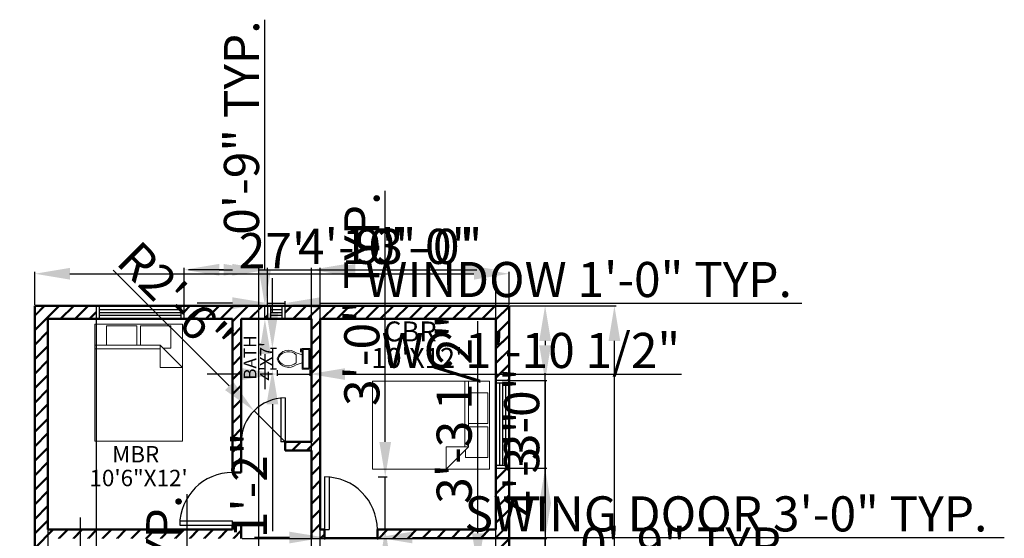
# Model space of a CAD drawing. Units: inches. Extents: x -584 to 444, y 228 to 1001.
# Tile 5 of 5: x -228 to 444, y 647 to 1001. Entities that reach past the tile are written whole.
import ezdxf

# ---------------------------------------------------------------- set-up
doc = ezdxf.new("R2010")
doc.units = ezdxf.units.IN
for name, color, linetype, lineweight in [('A-ANNO-DIMS', 2, 'Continuous', 18), ('A-AREA-IDEN', 7, 'Continuous', 25), ('A-DOOR', 3, 'Continuous', 25), ('A-FLOR-FIXT', 9, 'Continuous', 18), ('A-FURN', 8, 'Continuous', 18), ('A-GLAZ', 4, 'Continuous', 25), ('A-WALL', 7, 'Continuous', 50), ('A-WALL-PATT', 3, 'Continuous', 13)]:
    doc.layers.add(name, color=color, linetype=linetype, lineweight=lineweight)
doc.styles.get("Standard").update_dxf_attribs({"font": 'arial.ttf'})
doc.dimstyles.new('ISO-25', dxfattribs={"dimtxt": 24, "dimasz": 24, "dimexe": 1.25, "dimexo": 0.625, "dimtad": 1, "dimdec": 1, "dimlunit": 3, "dimtxsty": 'Standard', "dimcen": 2.5, "dimadec": 0, "dimazin": 0, "dimtfac": 1, "dimtdec": 1, "dimtmove": 0, "dimatfit": 3, "dimfxl": 1, "dimarcsym": 0})

# ---------------------------------------------------------------- blocks, each defined once
blk = doc.blocks.new('Bed - Queen')
for p, q in [((0, -80.00003), (0, 0)), ((0, 0), (59.99999, 0)), ((59.99999, 0), (59.99999, -80.00003)), ((7.99999, -1.2), (28.79998, -1.2)), ((7.99999, -14.4), (7.99999, -1.2)), ((28.79998, -1.2), (28.79998, -14.4)), ((31.19999, -1.2), (51.99999, -1.2)), ((31.19999, -14.4), (31.19999, -1.2)), ((51.99999, -1.2), (51.99999, -16.4)), ((0, -14.4), (44.8, -14.4)), ((44.8, -16.8), (0, -16.8)), ((59.99999, -29.6), (44.8, -14.4)), ((44.8, -14.4), (44.8, -29.6)), ((51.99999, -16.4), (46.79936, -16.4)), ((44.8, -29.6), (59.99999, -29.6)), ((59.99999, -80.00003), (0, -80.00003))]:
    blk.add_line(p, q)
blk = doc.blocks.new('Toilet - top')
for p, q in [((-10, -8.5), (-8, -8.5)), ((-10, -9.5), (-10, -8.5)), ((-7, -9.5), (-10, -9.5)), ((-8, -8.5), (-8, -8)), ((-7, -8), (-7, -9.5)), ((-4, -8), (-6, -14)), ((4, -8), (6, -14)), ((9.5, -6), (9.5, -2)), ((4, -14), (-4, -14))]:
    blk.add_line(p, q)
blk.add_lwpolyline([(10.5, -8), (10.5, 0), (-10.5, 0), (-10.5, -8)], close=True)
for points in [[(-9.5, -2), (-9.5, -6)], [(8.5, -1), (-8.5, -1)], [(-8.5, -7), (8.5, -7)]]:
    blk.add_lwpolyline(points)
for centre, radius, start, end in [((-8.62, -1.88), 0.884, 81.8699, 188.1301), ((-8.62, -6.12), 0.884, 171.8699, 278.1301), ((8.62, -1.88), 0.884, 351.8699, 98.1301), ((8.62, -6.12), 0.884, 261.8699, 8.1301), ((3.52, -21.58), 12.17, 141.46911, 247.97143), ((4.2, -21.82), 11.33, 136.36773, 238.94682), ((-3.52, -21.58), 12.17, 292.02843, 38.53071), ((-4.2, -21.82), 11.33, 301.05301, 43.63209), ((0, -27.88), 4, 245.73182, 294.26817), ((0, -29), 4, 254.86053, 285.13947)]:
    blk.add_arc(centre, radius, start, end)
blk = doc.blocks.new('*D6')
at = {"layer": 'A-ANNO-DIMS', "color": 0, "lineweight": -2, "transparency": 16777216}
for p, q in [((-218.14, 806.16), (-218.14, 828.68)), ((-194.14, 827.43), (81.86, 827.43)), ((105.86, 806.16), (105.86, 828.68))]:
    blk.add_line(p, q, dxfattribs=at)
at = {"layer": 'A-ANNO-DIMS', "color": 0, "transparency": 16777216}
for points in [[(-194.14, 831.43), (-194.14, 823.43), (-218.14, 827.43)], [(81.86, 831.43), (81.86, 823.43), (105.86, 827.43)]]:
    blk.add_solid(points, dxfattribs=at)
at = {"layer": 'Defpoints', "color": 0, "transparency": 16777216}
for p in [(105.86, 827.43), (-218.14, 805.54), (105.86, 805.54)]:
    blk.add_point(p, dxfattribs=at)
at = {"layer": 'A-ANNO-DIMS', "color": 0, "transparency": 16777216, "insert": (-56.14, 840.11), "char_height": 24, "attachment_point": 5}
blk.add_mtext("27'", dxfattribs=at)
blk = doc.blocks.new('*D7')
at = {"layer": 'A-ANNO-DIMS', "color": 0, "lineweight": -2, "transparency": 16777216}
for p, q in [((106.48, 805.54), (179.05, 805.54)), ((177.8, 409.54), (177.8, 781.54)), ((106.48, 385.54), (179.05, 385.54))]:
    blk.add_line(p, q, dxfattribs=at)
at = {"layer": 'A-ANNO-DIMS', "color": 0, "transparency": 16777216}
for points in [[(173.8, 781.54), (181.8, 781.54), (177.8, 805.54)], [(173.8, 409.54), (181.8, 409.54), (177.8, 385.54)]]:
    blk.add_solid(points, dxfattribs=at)
at = {"layer": 'Defpoints', "color": 0, "transparency": 16777216}
for p in [(105.86, 805.54), (177.8, 805.54), (105.86, 385.54)]:
    blk.add_point(p, dxfattribs=at)
at = {"layer": 'A-ANNO-DIMS', "color": 0, "transparency": 16777216, "insert": (164.91, 595.54), "char_height": 24, "attachment_point": 5, "rotation": 90}
blk.add_mtext("35'", dxfattribs=at)
blk = doc.blocks.new('WIN-60IN')
for p, q in [((60, 9), (0, 9)), ((0, 9), (0, 0)), ((2, 9), (2, 0)), ((58, 0), (58, 9)), ((60, 0), (60, 9)), ((0, 0), (60, 0)), ((2, 6.5), (58, 6.5)), ((2, 4.5), (58, 4.5)), ((2, 2.5), (58, 2.5))]:
    blk.add_line(p, q)
blk = doc.blocks.new('WIN-12IN')
for p, q in [((12, 9), (0, 9)), ((0, 9), (0, 0)), ((2, 9), (2, 0)), ((10, 0), (10, 9)), ((12, 0), (12, 9)), ((0, 0), (12, 0)), ((2, 6.5), (10, 6.5)), ((2, 4.5), (10, 4.5)), ((2, 2.5), (10, 2.5))]:
    blk.add_line(p, q)
blk = doc.blocks.new('DOOR-SWING-36IN')
for p, q in [((0, 36), (0, 0)), ((3, 36), (3, 0)), ((0, 0), (3, 0))]:
    blk.add_line(p, q)
blk.add_arc((0, 0), 36, 0, 90)
blk = doc.blocks.new('*D12')
at = {"layer": 'A-ANNO-DIMS', "color": 0, "lineweight": -2, "transparency": 16777216}
for p, q in [((72.86, 626.04), (48.86, 626.04)), ((96.86, 617.66), (96.86, 627.29)), ((96.86, 626.04), (105.86, 626.04)), ((105.86, 617.66), (105.86, 627.29)), ((129.86, 626.04), (301.4, 626.04))]:
    blk.add_line(p, q, dxfattribs=at)
at = {"layer": 'A-ANNO-DIMS', "color": 0, "transparency": 16777216}
for points in [[(72.86, 630.04), (72.86, 622.04), (96.86, 626.04)], [(129.86, 630.04), (129.86, 622.04), (105.86, 626.04)]]:
    blk.add_solid(points, dxfattribs=at)
at = {"layer": 'Defpoints', "color": 0, "transparency": 16777216}
for p in [(105.86, 626.04), (96.86, 617.04), (105.86, 617.04)]:
    blk.add_point(p, dxfattribs=at)
at = {"layer": 'A-ANNO-DIMS', "color": 0, "transparency": 16777216, "insert": (227.63, 638.92), "char_height": 24, "attachment_point": 5}
blk.add_mtext('0\'-9" TYP.', dxfattribs=at)
blk = doc.blocks.new('*D13')
at = {"layer": 'A-ANNO-DIMS', "color": 0, "lineweight": -2, "transparency": 16777216}
for p, q in [((-83.14, 807.34), (-107.14, 807.34)), ((-59.14, 806.16), (-59.14, 808.59)), ((-59.14, 807.34), (-47.14, 807.34)), ((-47.14, 806.16), (-47.14, 808.59)), ((-23.14, 807.34), (305.81, 807.34))]:
    blk.add_line(p, q, dxfattribs=at)
at = {"layer": 'A-ANNO-DIMS', "color": 0, "transparency": 16777216}
for points in [[(-83.14, 811.34), (-83.14, 803.34), (-59.14, 807.34)], [(-23.14, 811.34), (-23.14, 803.34), (-47.14, 807.34)]]:
    blk.add_solid(points, dxfattribs=at)
at = {"layer": 'Defpoints', "color": 0, "transparency": 16777216}
for p in [(-47.14, 807.34), (-59.14, 805.54), (-47.14, 805.54)]:
    blk.add_point(p, dxfattribs=at)
at = {"layer": 'A-ANNO-DIMS', "color": 0, "transparency": 16777216, "insert": (153.33, 820.38), "char_height": 24, "attachment_point": 5}
blk.add_mtext('WINDOW 1\'-0" TYP.', dxfattribs=at)
blk = doc.blocks.new('*D14')
at = {"layer": 'A-ANNO-DIMS', "color": 0, "lineweight": -2, "transparency": 16777216}
for p, q in [((-60.94, 829.54), (-60.94, 1001.08)), ((-59.77, 805.54), (-62.19, 805.54)), ((-60.94, 796.54), (-60.94, 805.54)), ((-59.77, 796.54), (-62.19, 796.54)), ((-60.94, 772.54), (-60.94, 748.54))]:
    blk.add_line(p, q, dxfattribs=at)
at = {"layer": 'A-ANNO-DIMS', "color": 0, "transparency": 16777216}
for points in [[(-64.94, 829.54), (-56.94, 829.54), (-60.94, 805.54)], [(-64.94, 772.54), (-56.94, 772.54), (-60.94, 796.54)]]:
    blk.add_solid(points, dxfattribs=at)
at = {"layer": 'Defpoints', "color": 0, "transparency": 16777216}
for p in [(-60.94, 805.54), (-59.14, 805.54), (-59.14, 796.54)]:
    blk.add_point(p, dxfattribs=at)
at = {"layer": 'A-ANNO-DIMS', "color": 0, "transparency": 16777216, "insert": (-73.82, 927.31), "char_height": 24, "attachment_point": 5, "rotation": 90}
blk.add_mtext('0\'-9" TYP.', dxfattribs=at)
blk = doc.blocks.new('*D16')
at = {"layer": 'A-ANNO-DIMS', "color": 0, "lineweight": -2, "transparency": 16777216}
for p, q in [((-114.06, 505.3), (-114.06, 676.85)), ((-125.44, 505.3), (-112.81, 505.3)), ((-114.06, 469.3), (-114.06, 481.3)), ((-125.44, 445.3), (-112.81, 445.3))]:
    blk.add_line(p, q, dxfattribs=at)
at = {"layer": 'A-ANNO-DIMS', "color": 0, "transparency": 16777216}
for points in [[(-118.06, 481.3), (-110.06, 481.3), (-114.06, 505.3)], [(-118.06, 469.3), (-110.06, 469.3), (-114.06, 445.3)]]:
    blk.add_solid(points, dxfattribs=at)
at = {"layer": 'Defpoints', "color": 0, "transparency": 16777216}
for p in [(-126.06, 505.3), (-114.06, 505.3), (-126.06, 445.3)]:
    blk.add_point(p, dxfattribs=at)
at = {"layer": 'A-ANNO-DIMS', "color": 0, "transparency": 16777216, "insert": (-126.94, 603.07), "char_height": 24, "attachment_point": 5, "rotation": 90}
blk.add_mtext('5\'-0" TYP.', dxfattribs=at)
blk = doc.blocks.new('*D17')
at = {"layer": 'A-ANNO-DIMS', "color": 0, "lineweight": -2, "transparency": 16777216}
for p, q in [((-44.14, 647.14), (-68.14, 647.14)), ((-20.14, 651.91), (-20.14, 645.89)), ((-20.14, 647.14), (15.86, 647.14)), ((15.86, 651.91), (15.86, 645.89)), ((39.86, 647.14), (444.11, 647.14))]:
    blk.add_line(p, q, dxfattribs=at)
at = {"layer": 'A-ANNO-DIMS', "color": 0, "transparency": 16777216}
for points in [[(-44.14, 651.14), (-44.14, 643.14), (-20.14, 647.14)], [(39.86, 651.14), (39.86, 643.14), (15.86, 647.14)]]:
    blk.add_solid(points, dxfattribs=at)
at = {"layer": 'Defpoints', "color": 0, "transparency": 16777216}
for p in [(-20.14, 652.54), (15.86, 652.54), (15.86, 647.14)]:
    blk.add_point(p, dxfattribs=at)
at = {"layer": 'A-ANNO-DIMS', "color": 0, "transparency": 16777216, "insert": (253.99, 660.19), "char_height": 24, "attachment_point": 5}
blk.add_mtext('SWING DOOR 3\'-0" TYP.', dxfattribs=at)
blk = doc.blocks.new('*D18')
at = {"layer": 'A-ANNO-DIMS', "color": 0, "lineweight": -2, "transparency": 16777216}
for p, q in [((21.26, 712.54), (21.26, 884.06)), ((16.48, 688.54), (22.51, 688.54)), ((21.26, 652.54), (21.26, 688.54)), ((16.48, 652.54), (22.51, 652.54)), ((21.26, 628.54), (21.26, 604.54))]:
    blk.add_line(p, q, dxfattribs=at)
at = {"layer": 'A-ANNO-DIMS', "color": 0, "transparency": 16777216}
for points in [[(17.26, 712.54), (25.26, 712.54), (21.26, 688.54)], [(17.26, 628.54), (25.26, 628.54), (21.26, 652.54)]]:
    blk.add_solid(points, dxfattribs=at)
at = {"layer": 'Defpoints', "color": 0, "transparency": 16777216}
for p in [(15.86, 688.54), (21.26, 688.54), (15.86, 652.54)]:
    blk.add_point(p, dxfattribs=at)
at = {"layer": 'A-ANNO-DIMS', "color": 0, "transparency": 16777216, "insert": (8.37, 810.3), "char_height": 24, "attachment_point": 5, "rotation": 90}
blk.add_mtext('3\'-0" TYP.', dxfattribs=at)
blk = doc.blocks.new('*D21')
at = {"layer": 'A-ANNO-DIMS', "color": 0, "lineweight": -2, "transparency": 16777216}
for p, q in [((-186.99, 636.91), (-186.99, 660.91)), ((-189.13, 612.91), (-185.74, 612.91)), ((-186.99, 612.91), (-186.99, 594.47)), ((-189.13, 594.47), (-185.74, 594.47)), ((-186.99, 570.47), (-186.99, 298.2))]:
    blk.add_line(p, q, dxfattribs=at)
at = {"layer": 'A-ANNO-DIMS', "color": 0, "transparency": 16777216}
for points in [[(-190.99, 636.91), (-182.99, 636.91), (-186.99, 612.91)], [(-190.99, 570.47), (-182.99, 570.47), (-186.99, 594.47)]]:
    blk.add_solid(points, dxfattribs=at)
at = {"layer": 'Defpoints', "color": 0, "transparency": 16777216}
for p in [(-189.76, 612.91), (-189.76, 594.47), (-186.99, 594.47)]:
    blk.add_point(p, dxfattribs=at)
at = {"layer": 'A-ANNO-DIMS', "color": 0, "transparency": 16777216, "insert": (-200.02, 422.34), "char_height": 24, "attachment_point": 5, "rotation": 90}
blk.add_mtext('RANGE 1\'-6 1/2"', dxfattribs=at)
blk = doc.blocks.new('*D23')
at = {"layer": 'A-ANNO-DIMS', "color": 0, "lineweight": -2, "transparency": 16777216}
for p, q in [((-52.47, 761.58), (-52.47, 757.61)), ((-30.15, 761.58), (-30.15, 757.61)), ((-76.47, 758.86), (-100.47, 758.86)), ((-52.47, 758.86), (-30.15, 758.86)), ((-6.15, 758.86), (223.63, 758.86))]:
    blk.add_line(p, q, dxfattribs=at)
at = {"layer": 'A-ANNO-DIMS', "color": 0, "transparency": 16777216}
for points in [[(-76.47, 762.86), (-76.47, 754.86), (-52.47, 758.86)], [(-6.15, 762.86), (-6.15, 754.86), (-30.15, 758.86)]]:
    blk.add_solid(points, dxfattribs=at)
at = {"layer": 'Defpoints', "color": 0, "transparency": 16777216}
for p in [(-52.47, 762.21), (-30.15, 762.21), (-30.15, 758.86)]:
    blk.add_point(p, dxfattribs=at)
at = {"layer": 'A-ANNO-DIMS', "color": 0, "transparency": 16777216, "insert": (120.74, 771.89), "char_height": 24, "attachment_point": 5}
blk.add_mtext('WC 1\'-10 1/2"', dxfattribs=at)
blk = doc.blocks.new('*D24')
at = {"layer": 'A-ANNO-DIMS', "color": 0, "lineweight": -2, "transparency": 16777216}
for p, q in [((-55.82, 800.4), (-55.82, 824.4)), ((-53.1, 776.4), (-57.07, 776.4)), ((-55.82, 776.4), (-55.82, 762.21)), ((-53.1, 762.21), (-57.07, 762.21)), ((-55.82, 738.21), (-55.82, 651.42))]:
    blk.add_line(p, q, dxfattribs=at)
at = {"layer": 'A-ANNO-DIMS', "color": 0, "transparency": 16777216}
for points in [[(-59.82, 800.4), (-51.82, 800.4), (-55.82, 776.4)], [(-59.82, 738.21), (-51.82, 738.21), (-55.82, 762.21)]]:
    blk.add_solid(points, dxfattribs=at)
at = {"layer": 'Defpoints', "color": 0, "transparency": 16777216}
for p in [(-52.47, 776.4), (-55.82, 762.21), (-52.47, 762.21)]:
    blk.add_point(p, dxfattribs=at)
at = {"layer": 'A-ANNO-DIMS', "color": 0, "transparency": 16777216, "insert": (-68.5, 682.81), "char_height": 24, "attachment_point": 5, "rotation": 90}
blk.add_mtext('1\'-2"', dxfattribs=at)
blk = doc.blocks.new('*D26')
at = {"layer": 'A-ANNO-DIMS', "color": 0, "lineweight": -2, "transparency": 16777216}
for p, q in [((84.51, 650.09), (84.51, 795.05)), ((75.37, 626.09), (85.76, 626.09)), ((84.51, 586.77), (84.51, 626.09)), ((75.37, 586.77), (85.76, 586.77)), ((84.51, 562.77), (84.51, 538.77))]:
    blk.add_line(p, q, dxfattribs=at)
at = {"layer": 'A-ANNO-DIMS', "color": 0, "transparency": 16777216}
for points in [[(80.51, 650.09), (88.51, 650.09), (84.51, 626.09)], [(80.51, 562.77), (88.51, 562.77), (84.51, 586.77)]]:
    blk.add_solid(points, dxfattribs=at)
at = {"layer": 'Defpoints', "color": 0, "transparency": 16777216}
for p in [(74.75, 626.09), (84.51, 626.09), (74.75, 586.77)]:
    blk.add_point(p, dxfattribs=at)
at = {"layer": 'A-ANNO-DIMS', "color": 0, "transparency": 16777216, "insert": (71.46, 734.57), "char_height": 24, "attachment_point": 5, "rotation": 90}
blk.add_mtext('3\'-3 1/2"', dxfattribs=at)
blk = doc.blocks.new('*D29')
at = {"layer": 'A-ANNO-DIMS', "color": 0, "lineweight": -2, "transparency": 16777216}
for p, q in [((-209.14, 795.91), (-209.14, 341.69)), ((-176.14, 795.91), (-176.14, 341.69)), ((-233.14, 342.94), (-257.14, 342.94)), ((-209.14, 342.94), (-176.14, 342.94)), ((-152.14, 342.94), (-62.69, 342.94))]:
    blk.add_line(p, q, dxfattribs=at)
at = {"layer": 'A-ANNO-DIMS', "color": 0, "transparency": 16777216}
for points in [[(-233.14, 346.94), (-233.14, 338.94), (-209.14, 342.94)], [(-152.14, 346.94), (-152.14, 338.94), (-176.14, 342.94)]]:
    blk.add_solid(points, dxfattribs=at)
at = {"layer": 'Defpoints', "color": 0, "transparency": 16777216}
for p in [(-209.14, 796.54), (-176.14, 796.54), (-176.14, 342.94)]:
    blk.add_point(p, dxfattribs=at)
at = {"layer": 'A-ANNO-DIMS', "color": 0, "transparency": 16777216, "insert": (-95.41, 355.82), "char_height": 24, "attachment_point": 5}
blk.add_mtext('2\'-9"', dxfattribs=at)
blk = doc.blocks.new('*D30')
at = {"layer": 'A-ANNO-DIMS', "color": 0, "lineweight": -2, "transparency": 16777216}
for p, q in [((-116.14, 806.16), (-116.14, 831.39)), ((-92.14, 830.14), (-83.14, 830.14)), ((-59.14, 806.16), (-59.14, 831.39)), ((-59.14, 830.14), (30.87, 830.14))]:
    blk.add_line(p, q, dxfattribs=at)
at = {"layer": 'A-ANNO-DIMS', "color": 0, "transparency": 16777216}
for points in [[(-92.14, 834.14), (-92.14, 826.14), (-116.14, 830.14)], [(-83.14, 834.14), (-83.14, 826.14), (-59.14, 830.14)]]:
    blk.add_solid(points, dxfattribs=at)
at = {"layer": 'Defpoints', "color": 0, "transparency": 16777216}
for p in [(-59.14, 830.14), (-116.14, 805.54), (-59.14, 805.54)]:
    blk.add_point(p, dxfattribs=at)
at = {"layer": 'A-ANNO-DIMS', "color": 0, "transparency": 16777216, "insert": (-2.14, 843.02), "char_height": 24, "attachment_point": 5}
blk.add_mtext('4\'-9"', dxfattribs=at)
blk = doc.blocks.new('*D31')
at = {"layer": 'A-ANNO-DIMS', "color": 0, "lineweight": -2, "transparency": 16777216}
for p, q in [((106.48, 805.54), (131.71, 805.54)), ((130.46, 781.54), (130.46, 778.54)), ((106.48, 754.54), (131.71, 754.54)), ((130.46, 754.54), (130.46, 664.52))]:
    blk.add_line(p, q, dxfattribs=at)
at = {"layer": 'A-ANNO-DIMS', "color": 0, "transparency": 16777216}
for points in [[(126.46, 781.54), (134.46, 781.54), (130.46, 805.54)], [(126.46, 778.54), (134.46, 778.54), (130.46, 754.54)]]:
    blk.add_solid(points, dxfattribs=at)
at = {"layer": 'Defpoints', "color": 0, "transparency": 16777216}
for p in [(105.86, 805.54), (105.86, 754.54), (130.46, 754.54)]:
    blk.add_point(p, dxfattribs=at)
at = {"layer": 'A-ANNO-DIMS', "color": 0, "transparency": 16777216, "insert": (117.57, 697.53), "char_height": 24, "attachment_point": 5, "rotation": 90}
blk.add_mtext('4\'-3"', dxfattribs=at)
blk = doc.blocks.new('*D32')
at = {"layer": 'A-ANNO-DIMS', "color": 0, "lineweight": -2, "transparency": 16777216}
for p, q in [((106.48, 694.54), (131.71, 694.54)), ((130.46, 670.54), (130.46, 641.04)), ((106.48, 617.04), (131.71, 617.04)), ((130.46, 617.04), (130.46, 471.93))]:
    blk.add_line(p, q, dxfattribs=at)
at = {"layer": 'A-ANNO-DIMS', "color": 0, "transparency": 16777216}
for points in [[(126.46, 670.54), (134.46, 670.54), (130.46, 694.54)], [(126.46, 641.04), (134.46, 641.04), (130.46, 617.04)]]:
    blk.add_solid(points, dxfattribs=at)
at = {"layer": 'Defpoints', "color": 0, "transparency": 16777216}
for p in [(105.86, 694.54), (105.86, 617.04), (130.46, 617.04)]:
    blk.add_point(p, dxfattribs=at)
at = {"layer": 'A-ANNO-DIMS', "color": 0, "transparency": 16777216, "insert": (117.42, 532.49), "char_height": 24, "attachment_point": 5, "rotation": 90}
blk.add_mtext('6\'-5 1/2"', dxfattribs=at)
blk = doc.blocks.new('*D36')
at = {"layer": 'A-ANNO-DIMS', "color": 0, "lineweight": -2, "transparency": 16777216}
for p, q in [((-23.14, 522.16), (-23.14, 831.39)), ((0.86, 830.14), (72.86, 830.14)), ((96.86, 522.16), (96.86, 831.39))]:
    blk.add_line(p, q, dxfattribs=at)
at = {"layer": 'A-ANNO-DIMS', "color": 0, "transparency": 16777216}
for points in [[(0.86, 834.14), (0.86, 826.14), (-23.14, 830.14)], [(72.86, 834.14), (72.86, 826.14), (96.86, 830.14)]]:
    blk.add_solid(points, dxfattribs=at)
at = {"layer": 'Defpoints', "color": 0, "transparency": 16777216}
for p in [(96.86, 830.14), (-23.14, 521.54), (96.86, 521.54)]:
    blk.add_point(p, dxfattribs=at)
at = {"layer": 'A-ANNO-DIMS', "color": 0, "transparency": 16777216, "insert": (36.86, 843.02), "char_height": 24, "attachment_point": 5}
blk.add_mtext('10\'-0"', dxfattribs=at)
blk = doc.blocks.new('*D40')
at = {"layer": 'A-ANNO-DIMS', "color": 0, "lineweight": -2, "transparency": 16777216}
for p, q in [((130.46, 670.54), (130.46, 759.57)), ((-76.52, 646.54), (131.71, 646.54)), ((130.46, 610.54), (130.46, 646.54)), ((-116.52, 610.54), (131.71, 610.54)), ((130.46, 586.54), (130.46, 562.54))]:
    blk.add_line(p, q, dxfattribs=at)
at = {"layer": 'A-ANNO-DIMS', "color": 0, "transparency": 16777216}
for points in [[(126.46, 670.54), (134.46, 670.54), (130.46, 646.54)], [(126.46, 586.54), (134.46, 586.54), (130.46, 610.54)]]:
    blk.add_solid(points, dxfattribs=at)
at = {"layer": 'Defpoints', "color": 0, "transparency": 16777216}
for p in [(-77.14, 646.54), (130.46, 646.54), (-117.14, 610.54)]:
    blk.add_point(p, dxfattribs=at)
at = {"layer": 'A-ANNO-DIMS', "color": 0, "transparency": 16777216, "insert": (117.57, 727.05), "char_height": 24, "attachment_point": 5, "rotation": 90}
blk.add_mtext('3\'-0"', dxfattribs=at)
blk = doc.blocks.new('*D41')
at = {"layer": 'A-ANNO-DIMS', "color": 0, "lineweight": -2, "transparency": 16777216}
for p, q in [((-89.14, 830.14), (-113.14, 830.14)), ((-65.14, 563.16), (-65.14, 831.39)), ((-65.14, 830.14), (-29.14, 830.14)), ((-29.14, 528.16), (-29.14, 831.39)), ((-5.14, 830.14), (83.89, 830.14))]:
    blk.add_line(p, q, dxfattribs=at)
at = {"layer": 'A-ANNO-DIMS', "color": 0, "transparency": 16777216}
for points in [[(-89.14, 834.14), (-89.14, 826.14), (-65.14, 830.14)], [(-5.14, 834.14), (-5.14, 826.14), (-29.14, 830.14)]]:
    blk.add_solid(points, dxfattribs=at)
at = {"layer": 'Defpoints', "color": 0, "transparency": 16777216}
for p in [(-29.14, 830.14), (-65.14, 562.54), (-29.14, 527.54)]:
    blk.add_point(p, dxfattribs=at)
at = {"layer": 'A-ANNO-DIMS', "color": 0, "transparency": 16777216, "insert": (51.37, 843.02), "char_height": 24, "attachment_point": 5}
blk.add_mtext('3\'-0"', dxfattribs=at)
blk = doc.blocks.new('*D42')
at = {"layer": 'A-ANNO-DIMS', "color": 0, "lineweight": -2, "transparency": 16777216}
for p, q in [((-164.54, 829.93), (-85.33, 750.72)), ((-47.14, 712.54), (-68.36, 733.75))]:
    blk.add_line(p, q, dxfattribs=at)
at = {"layer": 'A-ANNO-DIMS', "color": 0, "transparency": 16777216}
blk.add_solid([(-82.5, 753.55), (-88.16, 747.89), (-68.36, 733.75)], dxfattribs=at)
at = {"layer": 'Defpoints', "color": 0, "transparency": 16777216}
for p in [(-68.36, 733.75), (-47.14, 712.54)]:
    blk.add_point(p, dxfattribs=at)
at = {"layer": 'A-ANNO-DIMS', "color": 0, "transparency": 16777216, "insert": (-124.31, 807.92), "char_height": 24, "attachment_point": 5, "rotation": 315.00114}
blk.add_mtext('R2\'-6"', dxfattribs=at)

msp = doc.modelspace()

# ---------------------------------------------------------------- hatches: boundary and pattern name
at = {"layer": 'A-WALL-PATT'}
h = msp.add_hatch(dxfattribs=at)
h.set_pattern_fill('JIS_LC_8A', color=256, scale=0.9)
h.set_pattern_definition([(45, (105.857, 805.537), (-4.96389, 4.96389), []), (45, (106.757, 805.537), (-4.96389, 4.96389), [])])
h.paths.add_polyline_path([(105.86, 694.54), (96.86, 694.54), (96.86, 652.54), (15.86, 652.54), (15.86, 646.54), (96.86, 646.54), (96.86, 617.04), (105.86, 617.04)])
h.paths.add_polyline_path([(-77.14, 655.54), (-83.14, 655.54), (-83.14, 652.54), (-209.14, 652.54), (-209.14, 796.54), (-176.14, 796.54), (-176.14, 805.54), (-218.14, 805.54), (-218.14, 610.54), (-209.14, 610.54), (-209.14, 646.54), (-77.14, 646.54)])
h.paths.add_polyline_path([(-209.14, 598.54), (-218.14, 598.54), (-218.14, 505.54), (-209.14, 505.54), (-209.14, 556.54), (-111.14, 556.54), (-110.14, 556.54), (-110.14, 562.54), (-111.14, 562.54), (-111.14, 610.54), (-117.14, 610.54), (-117.14, 562.54), (-209.14, 562.54)])
h.paths.add_polyline_path([(-59.14, 805.54), (-116.14, 805.54), (-116.14, 796.54), (-83.14, 796.54), (-83.14, 691.54), (-77.14, 691.54), (-77.14, 796.54), (-59.14, 796.54)])
h.paths.add_polyline_path([(105.86, 805.54), (-47.14, 805.54), (-47.14, 796.54), (-29.14, 796.54), (-29.14, 712.54), (-47.14, 712.54), (-47.14, 706.54), (-29.14, 706.54), (-29.14, 646.54), (-20.14, 646.54), (-20.14, 652.54), (-23.14, 652.54), (-23.14, 796.54), (96.86, 796.54), (96.86, 754.54), (105.86, 754.54)])
h.paths.add_polyline_path([(-65.14, 385.54), (-65.14, 562.54), (-71.14, 562.54), (-74.14, 562.54), (-74.14, 556.54), (-71.14, 556.54), (-71.14, 394.54), (-209.14, 394.54), (-209.14, 445.54), (-218.14, 445.54), (-218.14, 385.54)])

# ---------------------------------------------------------------- linework, layer by layer
at = {"layer": 'A-DOOR'}
for p, q in [((-50.14, 742.54), (-50.14, 712.54)), ((-47.14, 742.54), (-47.14, 712.54)), ((-47.14, 712.54), (-50.14, 712.54))]:
    msp.add_line(p, q, dxfattribs=at)
msp.add_arc((-47.14, 712.54), 30, 90, 180, dxfattribs=at)
at = {"layer": 'A-WALL'}
for p, q in [((105.86, 805.54), (-218.14, 805.54)), ((-218.14, 805.54), (-218.14, 385.54)), ((105.86, 385.54), (105.86, 805.54)), ((-209.14, 796.54), (-209.14, 652.54)), ((-83.14, 796.54), (-209.14, 796.54)), ((-83.14, 796.54), (-83.14, 691.54)), ((-77.14, 796.54), (-77.14, 691.54)), ((-29.14, 796.54), (-77.14, 796.54)), ((-29.14, 796.54), (-29.14, 712.54)), ((96.86, 796.54), (-23.14, 796.54)), ((-23.14, 796.54), (-23.14, 652.54)), ((96.86, 652.54), (96.86, 796.54)), ((-29.14, 712.54), (-47.14, 712.54)), ((-47.14, 712.54), (-47.14, 706.54)), ((-29.14, 706.54), (-47.14, 706.54)), ((-29.14, 706.54), (-29.14, 646.54)), ((-77.14, 691.54), (-83.14, 691.54)), ((-83.14, 652.54), (-209.14, 652.54)), ((-77.14, 655.54), (-83.14, 655.54)), ((-83.14, 655.54), (-83.14, 652.54)), ((-77.14, 655.54), (-77.14, 646.54)), ((-20.14, 652.54), (-23.14, 652.54)), ((-20.14, 652.54), (-20.14, 646.54)), ((96.86, 652.54), (15.86, 652.54)), ((15.86, 652.54), (15.86, 646.54))]:
    msp.add_line(p, q, dxfattribs=at)

# ---------------------------------------------------------------- block references
at = {"layer": 'A-DOOR', "rotation": 90.00000000000007}
msp.add_blockref('DOOR-SWING-36IN', (-83.14, 655.54), dxfattribs=at)
at = {"layer": 'A-DOOR'}
msp.add_blockref('DOOR-SWING-36IN', (-20.14, 652.54), dxfattribs=at)
at = {"layer": 'A-FLOR-FIXT', "xscale": 0.6756608337803138, "yscale": 0.6756608337803138, "zscale": 0.6756608337803138, "rotation": 270}
msp.add_blockref('Toilet - top', (-30.15, 769.3), dxfattribs=at)
at = {"layer": 'A-FURN'}
msp.add_blockref('Bed - Queen', (-177.19, 792.98), dxfattribs=at)
at = {"layer": 'A-FURN', "rotation": 270}
msp.add_blockref('Bed - Queen', (92.45, 753.93), dxfattribs=at)
at = {"layer": 'A-GLAZ'}
for name, p in [('WIN-60IN', (-176.14, 796.54)), ('WIN-12IN', (-59.14, 796.54))]:
    msp.add_blockref(name, p, dxfattribs=at)
at = {"layer": 'A-GLAZ', "rotation": 270.0000000000002}
msp.add_blockref('WIN-60IN', (96.86, 754.54), dxfattribs=at)

# ---------------------------------------------------------------- texts
at = {"layer": 'A-AREA-IDEN', "attachment_point": 1}
for s, width, gutter_width, insert, char_height in [('CBR\\P ', 789.3556, 68.29, (20.45, 794.81), 13.657), ("10'X12'\\P ", 789.3556, 68.29, (11.72, 776.7), 13.657), ('MBR ', 648.8713, 56.13, (-165.32, 709.66), 11.227), ('10\'6"X12\'', 648.8713, 56.13, (-180.74, 693.44), 11.227)]:
    msp.add_mtext_dynamic_manual_height_columns(s, width=width, gutter_width=gutter_width, heights=[0], dxfattribs=dict(at, insert=insert, char_height=char_height))
at = {"layer": 'A-AREA-IDEN', "char_height": 8.59, "attachment_point": 1, "rotation": 90}
for s, insert in [('BATH ', (-75.4, 754.95)), ("4'X7'", (-64.31, 754.41))]:
    msp.add_mtext_dynamic_manual_height_columns(s, width=496.4661, gutter_width=42.95, heights=[0], dxfattribs=dict(at, insert=insert))

# ---------------------------------------------------------------- dimensions: what is measured, and where the dimension line sits
at = {"layer": 'A-ANNO-DIMS'}
for base, p1, p2, angle, text, picture, middle in [((-60.94, 805.54), (-59.14, 796.54), (-59.14, 805.54), 90, '<> TYP.', '*D14', (-73.82, 927.31)), ((21.26, 688.54), (15.86, 652.54), (15.86, 688.54), 90, '<> TYP.', '*D18', (8.37, 810.3)), ((-114.06, 505.3), (-126.06, 445.3), (-126.06, 505.3), 90, '<> TYP.', '*D16', (-126.94, 603.07)), ((-186.99, 594.47), (-189.76, 612.91), (-189.76, 594.47), 270, 'RANGE <>', '*D21', (-200.02, 422.34))]:
    dim = msp.add_linear_dim(base=base, p1=p1, p2=p2, angle=angle, text=text, dimstyle='ISO-25', override={"dimdec": 1, "dimlfac": 1, "dimrnd": 0, "dimzin": 1, "dimdsep": 46, "dimlunit": 4, "dimfrac": 2}, dxfattribs=at)
    dim.commit()
    dim.dimension.update_dxf_attribs({"geometry": picture, "text_midpoint": middle})
for base, p1, p2, text, picture, middle in [((-47.14, 807.34), (-59.14, 805.54), (-47.14, 805.54), 'WINDOW <> TYP.', '*D13', (153.33, 820.38)), ((-30.15, 758.86), (-52.47, 762.21), (-30.15, 762.21), 'WC <>', '*D23', (120.74, 771.89)), ((15.86, 647.14), (-20.14, 652.54), (15.86, 652.54), 'SWING DOOR <> TYP.', '*D17', (253.99, 660.19)), ((105.86, 626.04), (96.86, 617.04), (105.86, 617.04), '<> TYP.', '*D12', (227.63, 638.92))]:
    dim = msp.add_linear_dim(base=base, p1=p1, p2=p2, text=text, dimstyle='ISO-25', override={"dimdec": 1, "dimlfac": 1, "dimrnd": 0, "dimzin": 1, "dimdsep": 46, "dimlunit": 4, "dimfrac": 2}, dxfattribs=at)
    dim.commit()
    dim.dimension.update_dxf_attribs({"geometry": picture, "text_midpoint": middle})
for base, p1, p2, override, picture, middle in [((105.86, 827.43), (-218.14, 805.54), (105.86, 805.54), {"dimclrd": 0, "dimclre": 0, "dimclrt": 0}, '*D6', (-56.14, 840.11)), ((-59.14, 830.14), (-116.14, 805.54), (-59.14, 805.54), {"dimdec": 1, "dimlfac": 1, "dimrnd": 0, "dimzin": 1, "dimdsep": 46, "dimlunit": 4, "dimfrac": 2}, '*D30', (-2.14, 843.02)), ((-29.14, 830.14), (-65.14, 562.54), (-29.14, 527.54), {"dimdec": 1, "dimlfac": 1, "dimrnd": 0, "dimzin": 1, "dimdsep": 46, "dimlunit": 4, "dimfrac": 2}, '*D41', (51.37, 843.02)), ((96.86, 830.14), (-23.14, 521.54), (96.86, 521.54), {"dimdec": 1, "dimlfac": 1, "dimrnd": 0, "dimzin": 1, "dimdsep": 46, "dimlunit": 4, "dimfrac": 2}, '*D36', (36.86, 843.02)), ((-176.14, 342.94), (-209.14, 796.54), (-176.14, 796.54), {"dimdec": 1, "dimlfac": 1, "dimrnd": 0, "dimzin": 1, "dimdsep": 46, "dimlunit": 4, "dimfrac": 2}, '*D29', (-95.41, 355.82))]:
    dim = msp.add_linear_dim(base=base, p1=p1, p2=p2, dimstyle='ISO-25', override=override, dxfattribs=at)
    dim.commit()
    dim.dimension.update_dxf_attribs({"geometry": picture, "text_midpoint": middle})
dim = msp.add_radius_dim(center=(-47.14, 712.54), mpoint=(-68.36, 733.75), dimstyle='ISO-25', override={"dimdec": 1, "dimlfac": 1, "dimrnd": 0, "dimzin": 1, "dimdsep": 46, "dimlunit": 4, "dimfrac": 2}, dxfattribs=at)
dim.commit()
dim.dimension.update_dxf_attribs({"geometry": '*D42', "text_midpoint": (-124.31, 807.92)})
for base, p1, p2, angle, override, picture, middle in [((-55.82, 762.21), (-52.47, 776.4), (-52.47, 762.21), 270, {"dimdec": 1, "dimlfac": 1, "dimrnd": 0, "dimzin": 1, "dimdsep": 46, "dimlunit": 4, "dimfrac": 2}, '*D24', (-68.5, 682.81)), ((130.46, 754.54), (105.86, 805.54), (105.86, 754.54), 90, {"dimdec": 1, "dimlfac": 1, "dimrnd": 0, "dimzin": 1, "dimdsep": 46, "dimlunit": 4, "dimfrac": 2}, '*D31', (117.57, 697.53)), ((177.8, 805.54), (105.86, 385.54), (105.86, 805.54), 90, {"dimclrd": 0, "dimclre": 0, "dimclrt": 0}, '*D7', (164.91, 595.54)), ((84.51, 626.09), (74.75, 586.77), (74.75, 626.09), 90, {"dimdec": 1, "dimlfac": 1, "dimrnd": 0, "dimzin": 1, "dimdsep": 46, "dimlunit": 4, "dimfrac": 2}, '*D26', (71.46, 734.57)), ((130.46, 646.54), (-117.14, 610.54), (-77.14, 646.54), 90, {"dimdec": 1, "dimlfac": 1, "dimrnd": 0, "dimzin": 1, "dimdsep": 46, "dimlunit": 4, "dimfrac": 2}, '*D40', (117.57, 727.05)), ((130.46, 617.04), (105.86, 694.54), (105.86, 617.04), 90, {"dimdec": 1, "dimlfac": 1, "dimrnd": 0, "dimzin": 1, "dimdsep": 46, "dimlunit": 4, "dimfrac": 2}, '*D32', (117.42, 532.49))]:
    dim = msp.add_linear_dim(base=base, p1=p1, p2=p2, angle=angle, dimstyle='ISO-25', override=override, dxfattribs=at)
    dim.commit()
    dim.dimension.update_dxf_attribs({"geometry": picture, "text_midpoint": middle})

doc.saveas('drawing.dxf')
